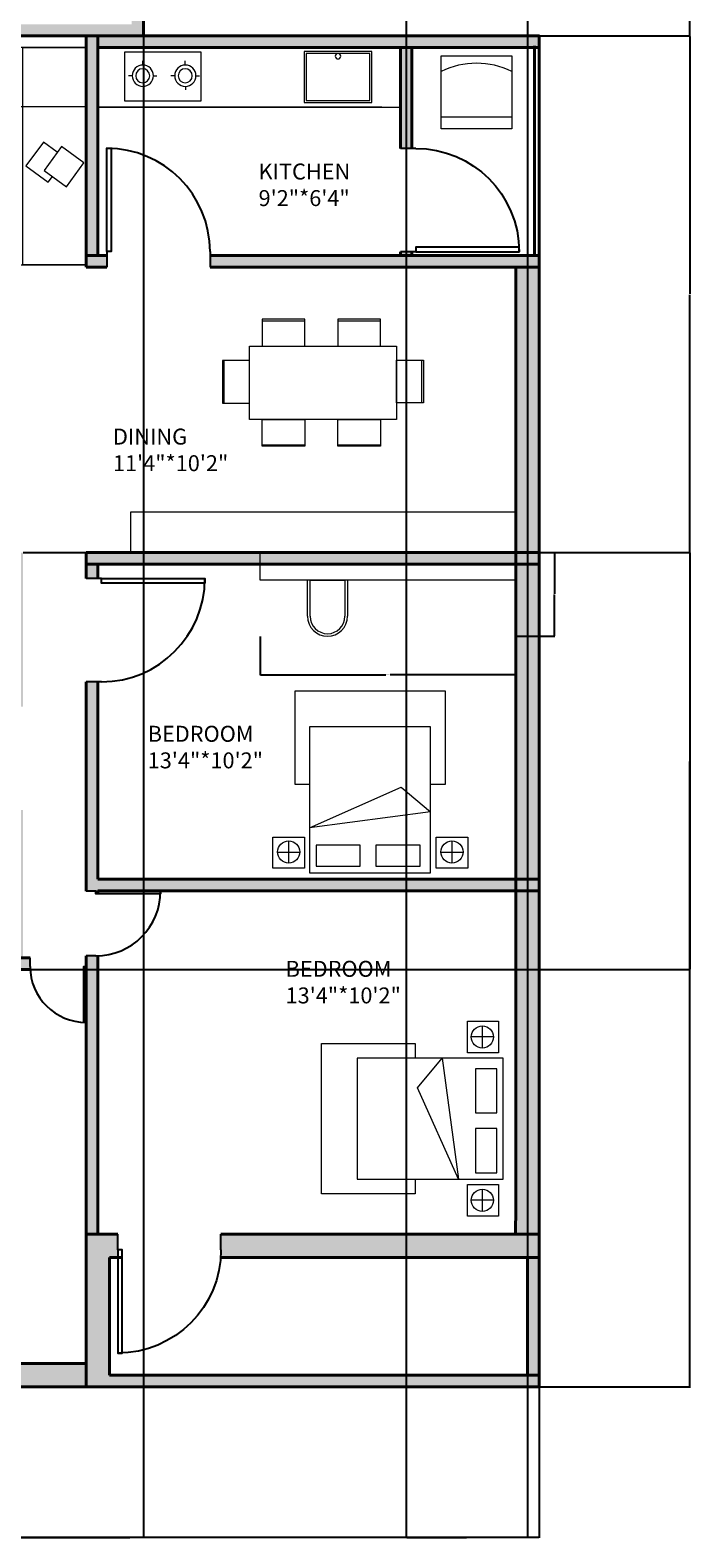
# Model space of a CAD drawing. Units: inches. Extents: x 1642 to 2399, y 1011 to 2291.
# Tile 3 of 7: x 2143 to 2399, y 1011 to 1595. Entities that reach past the tile are written whole.
import ezdxf

# ---------------------------------------------------------------- set-up
doc = ezdxf.new("R2010")
doc.units = ezdxf.units.IN
for name, color, linetype, lineweight in [('A-ANNO-DIMS', 2, 'Continuous', 18), ('A-AREA-IDEN', 7, 'Continuous', 20), ('A-DOOR', 4, 'Continuous', 25), ('A-EQPM', 8, 'Continuous', 18), ('A-FLOR-CASE', 30, 'Continuous', 18), ('A-FLOR-FIXT', 9, 'Continuous', 18), ('A-FURN', 8, 'Continuous', 18), ('A-WALL-PATT', 40, 'Continuous', 13), ('BED', 200, 'Continuous', 18), ('WALL', 40, 'Continuous', 40)]:
    doc.layers.add(name, color=color, linetype=linetype, lineweight=lineweight)
doc.styles.get("Standard").update_dxf_attribs({"font": 'arial.ttf'})
doc.dimstyles.get("Standard").update_dxf_attribs({"dimtxt": 0.18, "dimasz": 0.18, "dimexe": 0.18, "dimexo": 0.0625, "dimgap": 0.09, "dimtad": 0, "dimtih": 1, "dimtoh": 1, "dimdec": 4, "dimzin": 0, "dimdsep": 46, "dimtxsty": 'Standard', "dimcen": 0.09, "dimadec": 0, "dimazin": 0, "dimtfac": 1, "dimtdec": 4, "dimtofl": 0, "dimtmove": 0, "dimatfit": 3, "dimfxl": 1, "dimtolj": 1, "dimtzin": 0, "dimarcsym": 0})

# ---------------------------------------------------------------- blocks, each defined once
blk = doc.blocks.new('*U2')
for p, q in [((0, 0), (0, -6)), ((40, 0), (40, -6))]:
    blk.add_line(p, q)
blk.add_lwpolyline([(0, 0), (0, 40), (1.75, 40), (1.75, 0)], close=True)
blk.add_arc((0, 0), 40, 0, 90)
blk = doc.blocks.new('BED-DOUBLE-WITH-NIGHTSTANDS')
for p, q in [((8.62, 34.13), (8.62, 70.38)), ((8.62, 70.38), (66.79, 70.38)), ((66.79, 70.38), (66.79, 34.13)), ((14.22, 34.13), (8.62, 34.13)), ((14.22, 17.36), (49.69, 33.17)), ((49.69, 33.17), (61.11, 23.59)), ((66.79, 34.13), (61.11, 34.13)), ((61.11, 23.59), (14.22, 17.36)), ((6.17, 3.76), (6.17, 12.35)), ((69.41, 3.76), (69.41, 12.35)), ((1.82, 7.94), (10.42, 7.94)), ((65.06, 7.94), (73.65, 7.94))]:
    blk.add_line(p, q)
for points in [[(14.22, 0), (61.11, 0), (61.11, 56.52), (14.22, 56.52)], [(12.24, 1.79), (0, 1.79), (0, 13.82), (12.24, 13.82)], [(75.48, 1.79), (63.24, 1.79), (63.24, 13.82), (75.48, 13.82)], [(16.77, 2.51), (33.87, 2.51), (33.87, 10.66), (16.77, 10.66)], [(39.94, 2.51), (57.04, 2.51), (57.04, 10.66), (39.94, 10.66)]]:
    blk.add_lwpolyline(points, close=True)
for centre in [(6.12, 8.05), (69.36, 8.05)]:
    blk.add_circle(centre, 4.3)
blk = doc.blocks.new('TABLE-DINING-SIX-SEAT')
for p, q in [((15.31, 48.55), (31.81, 48.55)), ((44.68, 48.55), (61.18, 48.55)), ((0.59, 16.67), (0.59, 33.17)), ((77.22, 16.83), (77.22, 33.33)), ((15.31, 0.59), (31.81, 0.59)), ((44.68, 0.59), (61.18, 0.59))]:
    blk.add_line(p, q)
for points in [[(15.31, 38.77), (31.81, 38.77), (31.81, 49.15), (15.31, 49.15)], [(44.68, 38.77), (61.18, 38.77), (61.18, 49.15), (44.68, 49.15)], [(10.38, 38.77), (67.43, 38.77), (67.43, 10.38), (10.38, 10.38)], [(10.38, 16.67), (10.38, 33.17), (0, 33.17), (0, 16.67)], [(67.43, 16.83), (67.43, 33.33), (77.81, 33.33), (77.81, 16.83)], [(15.31, 10.38), (31.81, 10.38), (31.81, 0), (15.31, 0)], [(44.68, 10.38), (61.18, 10.38), (61.18, 0), (44.68, 0)]]:
    blk.add_lwpolyline(points, close=True)
blk = doc.blocks.new('SEATING-CORNER')
for points in [[(0, 84.13), (76.26, 84.13), (76.26, 61.34), (0, 61.34)], [(0, 0), (24.56, 0), (24.56, 84.13), (0, 84.13)], [(56.51, 80.66), (63.26, 71.39), (54.61, 65.09), (47.86, 74.37)], [(9.57, 45.8), (16.32, 36.53), (7.67, 30.23), (0.92, 39.51)]]:
    blk.add_lwpolyline(points, close=True)
for points in [[(58.1, 78.48), (63.51, 82.42), (70.26, 73.15), (61.61, 66.85), (60.02, 69.03)], [(11.16, 43.62), (16.57, 47.56), (23.32, 38.28), (14.67, 31.99), (13.08, 34.17)]]:
    blk.add_lwpolyline(points)
blk = doc.blocks.new('COOKTOP-TWO-BURNER')
for p, q in [((6.17, 13.89), (6.17, 15.59)), ((22.64, 13.89), (22.64, 15.59)), ((2, 9.67), (0.69, 9.67)), ((10.24, 9.72), (11.69, 9.72)), ((18.47, 9.67), (17.17, 9.67)), ((26.71, 9.72), (28.17, 9.72)), ((6.02, 5.65), (6.02, 4.35)), ((22.49, 5.65), (22.49, 4.35))]:
    blk.add_line(p, q)
blk.add_lwpolyline([(0, 18.89), (29.66, 18.89), (29.66, 0), (0, 0)], close=True)
for centre, radius in [((6.12, 9.77), 4.12), ((6.17, 9.77), 2.71), ((22.59, 9.77), 4.12), ((22.64, 9.77), 2.71)]:
    blk.add_circle(centre, radius)
blk = doc.blocks.new('SINK-KITCHEN-SINGLE')
for points in [[(0, 19.82), (26.24, 19.82), (26.24, 0), (0, 0)], [(0.83, 18.98), (25.41, 18.98), (25.41, 0.83), (0.83, 0.83)]]:
    blk.add_lwpolyline(points, close=True)
blk.add_circle((13.12, 17.93), 1.05)
blk = doc.blocks.new('UTILITY-APPLIANCE')
blk.add_line((0, 4.7), (27.35, 4.7))
blk.add_lwpolyline([(0, 28.26), (27.35, 28.26), (27.35, 0), (0, 0)], close=True)
blk.add_arc((13.68, -6.28), 31.65, 64.3994, 115.6006)
blk = doc.blocks.new('DESK-WITH-CHAIR')
blk.add_lwpolyline([(0, 32.44), (99.14, 32.44), (99.14, 21.72), (0, 21.72)], close=True)
for points in [[(18.41, 7.73), (18.41, 21.72)], [(19.41, 7.73), (19.41, 21.72), (32.87, 21.72), (32.87, 7.73)], [(33.87, 21.72), (33.87, 7.73)]]:
    blk.add_lwpolyline(points)
for radius in [7.73, 6.73]:
    blk.add_arc((26.14, 7.73), radius, 180, 0)
blk = doc.blocks.new('*D30')
at = {"layer": 'A-ANNO-DIMS', "color": 0, "lineweight": -2, "transparency": 16777216}
for p, q in [((2232.04, 1360.21), (2232.04, 1345.22)), ((2331.18, 1360.21), (2331.18, 1345.22)), ((2232.22, 1345.4), (2280.71, 1345.4)), ((2331, 1345.4), (2282.51, 1345.4))]:
    blk.add_line(p, q, dxfattribs=at)
at = {"layer": 'A-ANNO-DIMS', "color": 0, "transparency": 16777216}
for points in [[(2232.22, 1345.43), (2232.22, 1345.37), (2232.04, 1345.4)], [(2331, 1345.43), (2331, 1345.37), (2331.18, 1345.4)]]:
    blk.add_solid(points, dxfattribs=at)
at = {"layer": 'Defpoints', "color": 0, "transparency": 16777216}
for p in [(2232.04, 1360.27), (2331.18, 1360.27), (2331.18, 1345.4)]:
    blk.add_point(p, dxfattribs=at)
at = {"layer": 'A-ANNO-DIMS', "color": 0, "transparency": 16777216, "insert": (2281.61, 1345.4), "char_height": 0.18, "attachment_point": 5}
blk.add_mtext('\\A1;DESK 99 TYP.', dxfattribs=at)
blk = doc.blocks.new('*D31')
at = {"layer": 'A-ANNO-DIMS', "color": 0, "lineweight": -2, "transparency": 16777216}
for p, q in [((2331.24, 1392.71), (2346.23, 1392.71)), ((2346.05, 1392.53), (2346.05, 1376.67)), ((2346.05, 1360.45), (2346.05, 1376.31)), ((2331.24, 1360.27), (2346.23, 1360.27))]:
    blk.add_line(p, q, dxfattribs=at)
at = {"layer": 'A-ANNO-DIMS', "color": 0, "transparency": 16777216}
for points in [[(2346.02, 1392.53), (2346.08, 1392.53), (2346.05, 1392.71)], [(2346.02, 1360.45), (2346.08, 1360.45), (2346.05, 1360.27)]]:
    blk.add_solid(points, dxfattribs=at)
at = {"layer": 'Defpoints', "color": 0, "transparency": 16777216}
for p in [(2331.18, 1392.71), (2346.05, 1392.71), (2331.18, 1360.27)]:
    blk.add_point(p, dxfattribs=at)
at = {"layer": 'A-ANNO-DIMS', "color": 0, "transparency": 16777216, "insert": (2346.05, 1376.49), "char_height": 0.18, "attachment_point": 5}
blk.add_mtext('\\A1;32 TYP.', dxfattribs=at)
blk = doc.blocks.new('*D34')
at = {"layer": 'A-ANNO-DIMS', "color": 0, "lineweight": -2, "transparency": 16777216}
for p, q in [((2340.24, 1392.71), (2398.73, 1392.71)), ((2398.55, 1392.53), (2398.55, 1231.39)), ((2398.55, 1069.89), (2398.55, 1231.03)), ((2340.24, 1069.71), (2398.73, 1069.71))]:
    blk.add_line(p, q, dxfattribs=at)
at = {"layer": 'A-ANNO-DIMS', "color": 0, "transparency": 16777216}
for points in [[(2398.52, 1392.53), (2398.58, 1392.53), (2398.55, 1392.71)], [(2398.52, 1069.89), (2398.58, 1069.89), (2398.55, 1069.71)]]:
    blk.add_solid(points, dxfattribs=at)
at = {"layer": 'Defpoints', "color": 0, "transparency": 16777216}
for p in [(2340.18, 1392.71), (2398.55, 1392.71), (2340.18, 1069.71)]:
    blk.add_point(p, dxfattribs=at)
at = {"layer": 'A-ANNO-DIMS', "color": 0, "transparency": 16777216, "insert": (2398.55, 1231.21), "char_height": 0.18, "attachment_point": 5}
blk.add_mtext('\\A1;323', dxfattribs=at)
blk = doc.blocks.new('*D35')
at = {"layer": 'A-ANNO-DIMS', "color": 0, "lineweight": -2, "transparency": 16777216}
for p, q in [((2340.24, 1592.71), (2398.73, 1592.71)), ((2398.55, 1592.53), (2398.55, 1492.89)), ((2398.55, 1392.89), (2398.55, 1492.53)), ((2340.24, 1392.71), (2398.73, 1392.71))]:
    blk.add_line(p, q, dxfattribs=at)
at = {"layer": 'A-ANNO-DIMS', "color": 0, "transparency": 16777216}
for points in [[(2398.52, 1592.53), (2398.58, 1592.53), (2398.55, 1592.71)], [(2398.52, 1392.89), (2398.58, 1392.89), (2398.55, 1392.71)]]:
    blk.add_solid(points, dxfattribs=at)
at = {"layer": 'Defpoints', "color": 0, "transparency": 16777216}
for p in [(2340.18, 1592.71), (2398.55, 1592.71), (2340.18, 1392.71)]:
    blk.add_point(p, dxfattribs=at)
at = {"layer": 'A-ANNO-DIMS', "color": 0, "transparency": 16777216, "insert": (2398.55, 1492.71), "char_height": 0.18, "attachment_point": 5}
blk.add_mtext('\\A1;200', dxfattribs=at)
blk = doc.blocks.new('*D36')
at = {"layer": 'A-ANNO-DIMS', "color": 0, "lineweight": -2, "transparency": 16777216}
for p, q in [((2340.24, 1709.46), (2398.73, 1709.46)), ((2398.55, 1709.28), (2398.55, 1651.26)), ((2398.55, 1592.89), (2398.55, 1650.9)), ((2340.24, 1592.71), (2398.73, 1592.71))]:
    blk.add_line(p, q, dxfattribs=at)
at = {"layer": 'A-ANNO-DIMS', "color": 0, "transparency": 16777216}
for points in [[(2398.52, 1709.28), (2398.58, 1709.28), (2398.55, 1709.46)], [(2398.52, 1592.89), (2398.58, 1592.89), (2398.55, 1592.71)]]:
    blk.add_solid(points, dxfattribs=at)
at = {"layer": 'Defpoints', "color": 0, "transparency": 16777216}
for p in [(2340.18, 1709.46), (2398.55, 1709.46), (2340.18, 1592.71)]:
    blk.add_point(p, dxfattribs=at)
at = {"layer": 'A-ANNO-DIMS', "color": 0, "transparency": 16777216, "insert": (2398.55, 1651.08), "char_height": 0.18, "attachment_point": 5}
blk.add_mtext('\\A1;116.75', dxfattribs=at)
blk = doc.blocks.new('*D40')
at = {"layer": 'A-ANNO-DIMS', "color": 0, "lineweight": -2, "transparency": 16777216}
for p, q in [((1796.18, 1709.39), (1796.18, 1011.19)), ((2186.88, 1709.39), (2186.88, 1011.19)), ((1796.36, 1011.37), (1991.13, 1011.37)), ((2186.7, 1011.37), (1991.92, 1011.37))]:
    blk.add_line(p, q, dxfattribs=at)
at = {"layer": 'A-ANNO-DIMS', "color": 0, "transparency": 16777216}
for points in [[(1796.36, 1011.4), (1796.36, 1011.34), (1796.18, 1011.37)], [(2186.7, 1011.4), (2186.7, 1011.34), (2186.88, 1011.37)]]:
    blk.add_solid(points, dxfattribs=at)
at = {"layer": 'Defpoints', "color": 0, "transparency": 16777216}
for p in [(1796.18, 1709.46), (2186.88, 1709.46), (2186.88, 1011.37)]:
    blk.add_point(p, dxfattribs=at)
at = {"layer": 'A-ANNO-DIMS', "color": 0, "transparency": 16777216, "insert": (1991.53, 1011.37), "char_height": 0.18, "attachment_point": 5}
blk.add_mtext('\\A1;390.7', dxfattribs=at)
blk = doc.blocks.new('*D45')
at = {"layer": 'A-ANNO-DIMS', "color": 0, "lineweight": -2, "transparency": 16777216}
for p, q in [((2023.71, 1069.65), (2023.71, 1011.19)), ((2340.18, 1069.65), (2340.18, 1011.19)), ((2023.89, 1011.37), (2181.55, 1011.37)), ((2340, 1011.37), (2182.34, 1011.37))]:
    blk.add_line(p, q, dxfattribs=at)
at = {"layer": 'A-ANNO-DIMS', "color": 0, "transparency": 16777216}
for points in [[(2023.89, 1011.4), (2023.89, 1011.34), (2023.71, 1011.37)], [(2340, 1011.4), (2340, 1011.34), (2340.18, 1011.37)]]:
    blk.add_solid(points, dxfattribs=at)
at = {"layer": 'Defpoints', "color": 0, "transparency": 16777216}
for p in [(2023.71, 1069.71), (2340.18, 1069.71), (2340.18, 1011.37)]:
    blk.add_point(p, dxfattribs=at)
at = {"layer": 'A-ANNO-DIMS', "color": 0, "transparency": 16777216, "insert": (2181.95, 1011.37), "char_height": 0.18, "attachment_point": 5}
blk.add_mtext('\\A1;316.5', dxfattribs=at)
blk = doc.blocks.new('*D47')
at = {"layer": 'A-ANNO-DIMS', "color": 0, "lineweight": -2, "transparency": 16777216}
for p, q in [((2288.68, 1713.89), (2288.68, 1011.19)), ((2335.68, 1713.89), (2335.68, 1011.19)), ((2288.86, 1011.37), (2311.96, 1011.37)), ((2335.5, 1011.37), (2312.4, 1011.37))]:
    blk.add_line(p, q, dxfattribs=at)
at = {"layer": 'A-ANNO-DIMS', "color": 0, "transparency": 16777216}
for points in [[(2288.86, 1011.4), (2288.86, 1011.34), (2288.68, 1011.37)], [(2335.5, 1011.4), (2335.5, 1011.34), (2335.68, 1011.37)]]:
    blk.add_solid(points, dxfattribs=at)
at = {"layer": 'Defpoints', "color": 0, "transparency": 16777216}
for p in [(2288.68, 1713.96), (2335.68, 1713.96), (2335.68, 1011.37)]:
    blk.add_point(p, dxfattribs=at)
at = {"layer": 'A-ANNO-DIMS', "color": 0, "transparency": 16777216, "insert": (2312.18, 1011.37), "char_height": 0.18, "attachment_point": 5}
blk.add_mtext('\\A1;47', dxfattribs=at)
blk = doc.blocks.new('*D49')
at = {"layer": 'A-ANNO-DIMS', "color": 0, "lineweight": -2, "transparency": 16777216}
for p, q in [((2140.3, 1392.71), (2398.73, 1392.71)), ((2398.55, 1392.53), (2398.55, 1312.16)), ((2398.55, 1231.42), (2398.55, 1311.79)), ((2135.24, 1231.24), (2398.73, 1231.24))]:
    blk.add_line(p, q, dxfattribs=at)
at = {"layer": 'A-ANNO-DIMS', "color": 0, "transparency": 16777216}
for points in [[(2398.52, 1392.53), (2398.58, 1392.53), (2398.55, 1392.71)], [(2398.52, 1231.42), (2398.58, 1231.42), (2398.55, 1231.24)]]:
    blk.add_solid(points, dxfattribs=at)
at = {"layer": 'Defpoints', "color": 0, "transparency": 16777216}
for p in [(2140.24, 1392.71), (2135.18, 1231.24), (2398.55, 1231.24)]:
    blk.add_point(p, dxfattribs=at)
at = {"layer": 'A-ANNO-DIMS', "color": 0, "transparency": 16777216, "insert": (2398.55, 1311.98), "char_height": 0.18, "attachment_point": 5}
blk.add_mtext('\\A1;161.46', dxfattribs=at)

msp = doc.modelspace()

# ---------------------------------------------------------------- hatches: boundary and pattern name
at = {"layer": 'A-WALL-PATT'}
h = msp.add_hatch(color=256, dxfattribs=at)
h.dxf.hatch_style = 1
h.paths.add_polyline_path([(2340.1804, 2185.4562), (2211.0983, 2185.4562, -0.01876983), (2211.211, 2182.4562), (2211.211, 2176.4562), (2331.211, 2176.4562), (2331.211, 2043.4562), (2171.211, 2043.4562), (2171.211, 2038.9562), (2331.211, 2038.9562), (2331.211, 1916.9562), (2171.211, 1916.9562), (2171.211, 1918.9365), (2166.711, 1918.9365), (2166.711, 1912.4562), (2340.1804, 1912.4562)])
h.paths.add_polyline_path([(2171.211, 2043.4562), (2171.211, 2043.9025), (2170.5217, 2043.9025), (2166.711, 2043.9025), (2166.711, 2038.9562), (2166.711, 1958.9365), (2171.211, 1958.9365)], flags=17)
h.paths.add_polyline_path([(2129.211, 1971.5979), (2124.711, 1971.5979), (2124.711, 1918.4562), (2067.711, 1918.4562), (2067.711, 1913.9562), (2129.211, 1913.9562)])
h.paths.add_polyline_path([(2067.711, 2015.4562), (2124.711, 2015.4562), (2124.711, 2019.9562), (2058.711, 2019.9562), (2058.711, 2015.4562), (2058.711, 1922.9562), (1982.211, 1922.9562), (1982.211, 2015.4562), (1982.211, 2019.9562), (1916.211, 2019.9562), (1916.211, 2070.9562), (1911.711, 2070.9562), (1911.711, 2015.4562), (1911.711, 2012.302), (1916.211, 2012.302), (1916.211, 2015.4562), (1973.211, 2015.4562), (1973.211, 1918.4562), (1973.211, 1913.9562), (2017.1804, 1913.9562), (2067.711, 1913.9562), (2067.711, 1918.4562)])
h.paths.add_polyline_path([(2131.1386, 2075.4562), (2118.1934, 2075.4562), (2118.1934, 2070.9562), (2131.1386, 2070.9562)], flags=17)
h.paths.add_polyline_path([(1918.8034, 2075.4562), (1909.4956, 2075.4562), (1909.4956, 2070.9562), (1918.8034, 2070.9562)], flags=17)
h.paths.add_polyline_path([(1874.211, 2029.9562), (1869.711, 2029.9562), (1869.711, 1960.7404), (1874.211, 1960.7404)], flags=17)
h.paths.add_polyline_path([(1916.211, 1972.302), (1911.711, 1972.302), (1911.711, 1918.4562), (1916.211, 1918.4562)], flags=17)
h.paths.add_polyline_path([(2340.1804, 1912.4562), (2331.1804, 1912.4562), (2331.1804, 1794.4562), (2210.1804, 1794.4562), (2210.1804, 1789.9562), (2279.6804, 1789.9562), (2340.1804, 1789.9562)])
h.paths.add_polyline_path([(2288.6804, 1789.9562), (2279.6804, 1789.9562), (2279.6804, 1785.0846), (2285.6804, 1785.0846), (2288.6804, 1785.0846)], flags=17)
h.paths.add_polyline_path([(2169.6804, 1789.9562), (2170.1804, 1789.9562), (2170.1804, 1794.4562), (2165.1804, 1794.4562), (2165.1804, 1713.9562), (2165.1804, 1709.4562), (2279.6804, 1709.4562), (2279.6804, 1718.4562), (2169.6804, 1718.4562)])
h.paths.add_polyline_path([(2288.6804, 1745.1973, -0.01876983), (2285.6804, 1745.0846), (2279.6804, 1745.0846), (2279.6804, 1709.4562), (2340.1804, 1709.4562), (2340.1804, 1789.9562), (2335.6804, 1789.9562), (2335.6804, 1713.9562), (2288.6804, 1713.9562)])
h.paths.add_polyline_path([(2165.1804, 1713.9562), (2140.6229, 1713.9562), (2088.923, 1713.9562), (2069.7509, 1713.9562), (2060.4457, 1713.9562), (2060.4457, 1709.4562), (2165.1804, 1709.4562)])
h.paths.add_polyline_path([(2020.4457, 1713.9562), (2017.1804, 1713.9562), (2012.6804, 1713.9562), (2009.1946, 1713.9562), (2009.1946, 1709.4562), (2020.4457, 1709.4562)])
h.paths.add_polyline_path([(1969.1946, 1713.9562), (1864.6804, 1713.9562), (1864.6804, 1798.9562), (1860.1804, 1798.9562), (1860.1804, 1792.9562), (1860.1804, 1752.9562), (1860.1804, 1718.4562), (1750.1804, 1718.4562), (1750.1804, 1749.2419), (1744.1804, 1749.2419, -0.01876983), (1741.1804, 1749.3546), (1741.1804, 1709.4562), (1969.1946, 1709.4562)])
h.paths.add_polyline_path([(1741.1804, 1803.4562), (1700.711, 1803.4562), (1700.711, 1794.4562), (1741.1804, 1794.4562)])
h.paths.add_polyline_path([(1820.1804, 1798.9562), (1741.1804, 1798.9562), (1741.1804, 1794.4562), (1741.1804, 1790.0365), (1741.1804, 1789.2419), (1744.1804, 1789.2419), (1750.1804, 1789.2419), (1750.1804, 1794.4562), (1820.1804, 1794.4562)], flags=17)
h.paths.add_polyline_path([(1800.6804, 1709.4562), (1796.1804, 1709.4562), (1796.1804, 1592.7078), (1978.9325, 1592.7078), (1978.9325, 1597.2078), (1800.6804, 1597.2078)])
h.paths.add_polyline_path([(2097.0678, 1709.4562), (2088.0678, 1709.4562), (2088.0678, 1599.6874), (2088.0678, 1597.2078), (2097.0678, 1597.2078)], flags=17)
h.paths.add_polyline_path([(2186.8766, 1709.4562), (2182.3766, 1709.4562), (2182.3766, 1597.2078), (2071.4624, 1597.2078), (2071.4624, 1592.7078), (2186.8766, 1592.7078)])
h.paths.add_polyline_path([(2078.1934, 2075.4562), (2022.711, 2075.4562), (2022.711, 2223.4562), (2166.711, 2223.4562), (2166.711, 2075.4562), (2166.711, 2070.9562), (2171.211, 2070.9562), (2171.211, 2138.8919), (2171.211, 2227.9562), (2335.711, 2227.9562), (2335.711, 2185.4562), (2340.1804, 2185.4562), (2340.1804, 2232.4562), (1874.211, 2232.4562), (1874.211, 2223.4562), (2018.211, 2223.4562), (2018.211, 2075.4562), (1958.8034, 2075.4562), (1958.8034, 2070.9562), (2018.211, 2070.9562), (2018.211, 2019.9562), (1982.211, 2019.9562), (1982.211, 2015.4562), (1982.211, 2010.9562), (2058.711, 2010.9562), (2058.711, 2015.4562), (2058.711, 2019.9562), (2022.711, 2019.9562), (2022.711, 2070.9562), (2078.1934, 2070.9562)])
h.paths.add_polyline_path([(1874.211, 2171.9562), (1874.211, 2176.4562), (1861.9371, 2176.4562), (1861.9371, 2173.4562), (1861.9371, 2167.4562), (1869.711, 2167.4562), (1869.711, 2069.7602), (1874.211, 2069.7602)], flags=17)
h.paths.add_polyline_path([(1705.211, 2227.9562), (1865.211, 2227.9562), (1865.211, 2176.4562), (1874.211, 2176.4562), (1874.211, 2232.4562), (1700.711, 2232.4562), (1700.711, 2176.4562), (1705.211, 2176.4562)])
h.paths.add_polyline_path([(1709.711, 2167.4562), (1821.9371, 2167.4562), (1821.9371, 2173.4562, -0.01876983), (1822.0498, 2176.4562), (1700.711, 2176.4562), (1700.711, 1913.9562), (1860.1804, 1913.9562), (1864.6804, 1913.9562), (1973.211, 1913.9562), (1973.211, 1918.4562), (1916.211, 1918.4562), (1874.211, 1918.4562), (1874.211, 1920.7404), (1869.711, 1920.7404), (1869.711, 1918.4562), (1860.1804, 1918.4562), (1709.711, 1918.4562), (1709.711, 2029.9562), (1874.211, 2029.9562), (1874.211, 2037.0364), (1869.711, 2037.0364), (1869.711, 2034.4562), (1709.711, 2034.4562)])
h.paths.add_polyline_path([(2017.1804, 1913.9562), (2012.6804, 1913.9562), (2012.6804, 1713.9562), (2017.1804, 1713.9562)])
h.paths.add_polyline_path([(1952.4341, 2110.3716), (2000.4134, 2110.3716), (2000.4134, 2133.4189), (1952.4341, 2133.4189)], flags=25)
h.paths.add_polyline_path([(2042.3983, 2110.7121), (2090.3775, 2110.7121), (2090.3775, 2133.7594), (2042.3983, 2133.7594)], flags=25)
h.paths.add_polyline_path([(2201.7332, 2091.8715), (2249.7125, 2091.8715), (2249.7125, 2114.9188), (2201.7332, 2114.9188)], flags=25)
h.paths.add_polyline_path([(1805.186, 2077.6915), (1853.1653, 2077.6915), (1853.1653, 2100.7388), (1805.186, 2100.7388)], flags=25)
h.paths.add_polyline_path([(1794.8897, 1974.6584), (1842.869, 1974.6584), (1842.869, 1997.7057), (1794.8897, 1997.7057)], flags=25)
h.paths.add_polyline_path([(2229.1796, 2204.4209), (2315.1362, 2204.4209), (2315.1362, 2217.1488), (2229.1796, 2217.1488)], flags=25)
h.paths.add_polyline_path([(1715.2159, 2199.5328), (1801.1724, 2199.5328), (1801.1724, 2212.2607), (1715.2159, 2212.2607)], flags=25)
h.paths.add_polyline_path([(2230.7681, 1755.7109), (2271.7283, 1755.7109), (2271.7283, 1778.7582), (2230.7681, 1778.7582)], flags=25)
h.paths.add_polyline_path([(1763.4713, 1764.1742), (1804.4315, 1764.1742), (1804.4315, 1787.2215), (1763.4713, 1787.2215)], flags=25)
h.paths.add_polyline_path([(2076.2643, 1955.0495), (2111.326, 1955.0495), (2111.326, 1978.0968), (2076.2643, 1978.0968)], flags=25)
h.paths.add_polyline_path([(1932.854, 1956.1217), (1967.9158, 1956.1217), (1967.9158, 1979.169), (1932.854, 1979.169)], flags=25)
h.paths.add_polyline_path([(2048.1203, 2031.6107), (2083.1821, 2031.6107), (2083.1821, 2054.658), (2048.1203, 2054.658)], flags=25)
h.paths.add_polyline_path([(2163.5754, 1863.7569), (2208.2347, 1863.7569), (2208.2347, 1886.8042), (2163.5754, 1886.8042)], flags=9)
h.paths.add_polyline_path([(2039.9286, 1809.0957), (2084.5879, 1809.0957), (2084.5879, 1832.143), (2039.9286, 1832.143)], flags=9)
h.paths.add_polyline_path([(1901.0045, 1814.0452), (1945.6638, 1814.0452), (1945.6638, 1837.0925), (1901.0045, 1837.0925)], flags=9)
h.paths.add_polyline_path([(1833.7282, 1852.5627), (1878.3875, 1852.5627), (1878.3875, 1875.61), (1833.7282, 1875.61)], flags=9)
h.paths.add_polyline_path([(2219.1375, 1926.2139), (2267.1167, 1926.2139), (2267.1167, 1949.2612), (2219.1375, 1949.2612)], flags=25)
h.paths.add_polyline_path([(1956.9598, 2029.7735), (1992.0216, 2029.7735), (1992.0216, 2052.8208), (1956.9598, 2052.8208)], flags=25)
h.paths.add_polyline_path([(2229.3, 1523.3399), (2270.2602, 1523.3399), (2270.2602, 1546.3872), (2229.3, 1546.3872)], flags=9)
h.paths.add_polyline_path([(1772.3039, 1526.9922), (1813.2641, 1526.9922), (1813.2641, 1550.0394), (1772.3039, 1550.0394)], flags=9)
h.paths.add_polyline_path([(2172.587, 1420.6999), (2217.2463, 1420.6999), (2217.2463, 1443.7472), (2172.587, 1443.7472)], flags=9)
h.paths.add_polyline_path([(1814.3549, 1422.215), (1859.0143, 1422.215), (1859.0143, 1445.2623), (1814.3549, 1445.2623)], flags=9)
h.paths.add_polyline_path([(2186.0372, 1305.6227), (2234.0165, 1305.6227), (2234.0165, 1328.67), (2186.0372, 1328.67)], flags=9)
h.paths.add_polyline_path([(1756.747, 1349.0694), (1804.7263, 1349.0694), (1804.7263, 1372.1167), (1756.747, 1372.1167)], flags=9)
h.paths.add_polyline_path([(2239.449, 1214.6184), (2287.4282, 1214.6184), (2287.4282, 1237.6657), (2239.449, 1237.6657)], flags=9)
h.paths.add_polyline_path([(1767.104, 1213.8348), (1815.0832, 1213.8348), (1815.0832, 1236.8821), (1767.104, 1236.8821)], flags=9)
h.paths.add_polyline_path([(2046.6809, 1183.6854), (2094.6602, 1183.6854), (2094.6602, 1206.7327), (2046.6809, 1206.7327)], flags=9)
h.paths.add_polyline_path([(1947.2155, 1183.6854), (1995.1948, 1183.6854), (1995.1948, 1206.7327), (1947.2155, 1206.7327)], flags=9)
h.paths.add_polyline_path([(1959.3556, 1258.7871), (1994.4174, 1258.7871), (1994.4174, 1281.8344), (1959.3556, 1281.8344)], flags=9)
h.paths.add_polyline_path([(2049.6419, 1248.9629), (2084.7036, 1248.9629), (2084.7036, 1272.0102), (2049.6419, 1272.0102)], flags=9)
h.paths.add_polyline_path([(2092.7532, 1327.4852), (2127.815, 1327.4852), (2127.815, 1350.5325), (2092.7532, 1350.5325)], flags=9)
h.paths.add_polyline_path([(1944.9358, 1327.4852), (1979.9976, 1327.4852), (1979.9976, 1350.5325), (1944.9358, 1350.5325)], flags=9)
h.paths.add_polyline_path([(1974.5055, 1650.063), (2006.3695, 1650.063), (2006.3695, 1662.7909), (1974.5055, 1662.7909)], flags=9)
h = msp.add_hatch(color=256, dxfattribs=at)
h.dxf.hatch_style = 1
h.paths.add_polyline_path([(2078.7415, 1388.2078), (2028.211, 1388.2078), (2028.211, 1383.7078), (2069.7415, 1383.7078), (2069.7415, 1291.2078), (2069.7415, 1286.7078), (2135.7415, 1286.7078), (2135.7415, 1291.2078), (2078.7415, 1291.2078)])
h.paths.add_polyline_path([(1993.2415, 1383.7078), (2023.711, 1383.7078), (2023.711, 1388.2078), (1984.2415, 1388.2078), (1984.2415, 1291.2078), (1927.2415, 1291.2078), (1927.2415, 1296.6705), (1922.7415, 1296.6705), (1922.7415, 1291.2078), (1922.7415, 1235.7078), (1927.2415, 1235.7078), (1927.2415, 1237.2428), (1927.2415, 1277.2428), (1927.2415, 1286.7078), (1993.2415, 1286.7078), (1993.2415, 1291.2078)])
h.paths.add_polyline_path([(1927.2415, 1388.2078), (1922.7415, 1388.2078), (1922.7415, 1336.6705), (1927.2415, 1336.6705)])
h.paths.add_polyline_path([(1984.2415, 1392.7078), (1922.7415, 1392.7078), (1922.7415, 1388.2078), (1984.2415, 1388.2078)])
h.paths.add_polyline_path([(2023.711, 1392.7078), (1984.2415, 1392.7078), (1984.2415, 1388.2078), (2023.711, 1388.2078)])
h.paths.add_polyline_path([(2078.7415, 1392.7078), (2028.211, 1392.7078), (2028.211, 1388.2078), (2078.7415, 1388.2078)])
h.paths.add_polyline_path([(2140.2415, 1392.7078), (2078.7415, 1392.7078), (2078.7415, 1388.2078), (2135.7415, 1388.2078), (2140.2415, 1388.2078)])
h.paths.add_polyline_path([(2028.211, 1592.7078), (2023.711, 1592.7078), (2023.711, 1392.7078), (2028.211, 1392.7078)])
h.paths.add_polyline_path([(2028.211, 1388.2078), (2023.711, 1388.2078), (2023.711, 1383.7078), (2028.211, 1383.7078)])
h.paths.add_polyline_path([(2028.211, 1392.7078), (2023.711, 1392.7078), (2023.711, 1388.2078), (2028.211, 1388.2078)])
h.paths.add_polyline_path([(2140.2415, 1388.2078), (2135.7415, 1388.2078), (2135.7415, 1332.9578), (2140.2415, 1332.9578)])
h.paths.add_polyline_path([(2069.7415, 1291.2078), (2069.7415, 1295.7078), (2028.211, 1295.7078), (2023.711, 1295.7078), (1993.2415, 1295.7078), (1993.2415, 1291.2078), (1993.2415, 1286.7078), (2029.2415, 1286.7078), (2047.9002, 1286.7078), (2053.9738, 1286.7078), (2069.7415, 1286.7078)])
h.paths.add_polyline_path([(2140.2415, 1291.2078), (2140.2415, 1292.9578), (2135.7415, 1292.9578), (2135.7415, 1269.1323), (2135.7415, 1235.7078), (2140.2415, 1235.7078)])
h.paths.add_polyline_path([(2232.0378, 1392.7078), (2164.6804, 1392.7078), (2164.6804, 1388.2078), (2232.0378, 1388.2078)])
h.paths.add_polyline_path([(2331.1804, 1392.7078), (2232.0378, 1392.7078), (2232.0378, 1388.2078), (2331.1804, 1388.2078)])
h.paths.add_polyline_path([(2340.1804, 1392.7078), (2331.1804, 1392.7078), (2331.1804, 1388.2078), (2340.1804, 1388.2078)])
h.paths.add_polyline_path([(2340.1804, 1388.2078), (2331.1804, 1388.2078), (2331.1804, 1381.9887), (2331.1804, 1266.2078), (2340.1804, 1266.2078)])
h.paths.add_polyline_path([(2331.1804, 1266.2078), (2169.1804, 1266.2078), (2169.1804, 1342.6266), (2164.6804, 1342.6266), (2164.6804, 1266.2078), (2164.6804, 1261.6393), (2168.4442, 1261.6393), (2169.1804, 1261.6393), (2169.1804, 1261.7078), (2331.1804, 1261.7078)])
h.paths.add_polyline_path([(2340.1804, 1266.2078), (2331.1804, 1266.2078), (2331.1804, 1261.7078), (2340.1804, 1261.7078)])
h.paths.add_polyline_path([(2340.1804, 1503.2078), (2331.1804, 1503.2078), (2331.1804, 1392.7078), (2340.1804, 1392.7078)])
h.paths.add_polyline_path([(2340.1804, 1261.7078), (2331.1804, 1261.7078), (2331.1804, 1139.2078), (2331.0462, 1128.7078), (2340.1804, 1128.7078)])
h.paths.add_polyline_path([(2169.1804, 1236.5578, -0.00733557), (2168.4442, 1236.547), (2164.6804, 1236.547), (2164.6804, 1128.7078), (2169.1804, 1128.7078)])
h.paths.add_polyline_path([(2095.1813, 1235.7078), (2028.211, 1235.7078), (2028.211, 1231.2428), (2095.1813, 1231.2428)])
h.paths.add_polyline_path([(2028.211, 1286.7078), (2023.711, 1286.7078), (2023.711, 1235.7078), (2028.211, 1235.7078)])
h.paths.add_polyline_path([(2028.211, 1235.7078), (2023.711, 1235.7078), (2023.711, 1231.2428), (2028.211, 1231.2428)])
h.paths.add_polyline_path([(2023.711, 1235.7078), (1967.2415, 1235.7078), (1967.2415, 1231.2428), (2023.711, 1231.2428)])
h.paths.add_polyline_path([(2028.211, 1231.2428), (2023.711, 1231.2428), (2023.711, 1078.7078), (2028.211, 1078.7078)])
h.paths.add_polyline_path([(1866.711, 1074.2078), (1705.211, 1074.2078), (1705.211, 1119.7078), (1700.711, 1119.7078), (1700.711, 1069.7078), (1866.711, 1069.7078)])
h.paths.add_polyline_path([(2023.711, 1078.7078), (1875.711, 1078.7078), (1875.711, 1074.2078), (1875.711, 1069.7078), (2023.711, 1069.7078)])
h.paths.add_polyline_path([(2028.211, 1078.7078), (2023.711, 1078.7078), (2023.711, 1069.7078), (2028.211, 1069.7078)])
h.paths.add_polyline_path([(2164.6804, 1078.7078), (2028.211, 1078.7078), (2028.211, 1069.7078), (2164.6804, 1069.7078), (2164.6804, 1074.2078)])
h = msp.add_hatch(color=256, dxfattribs=at)
h.dxf.hatch_style = 1
h.paths.add_polyline_path([(1875.711, 1343.4643), (1871.211, 1343.4643), (1871.211, 1266.2078), (1709.711, 1266.2078), (1709.711, 1388.2078), (1700.711, 1388.2078), (1700.711, 1261.7078), (1709.711, 1261.7078), (1875.711, 1261.7078)])
h.paths.add_polyline_path([(1761.211, 1583.7078), (1761.211, 1588.2078), (1761.211, 1592.7078), (1700.711, 1592.7078), (1700.711, 1388.2078), (1709.711, 1388.2078), (1808.8535, 1388.2078), (1871.211, 1388.2078), (1871.211, 1397.2078), (1709.711, 1397.2078), (1709.711, 1503.2078), (1761.211, 1503.2078), (1825.4443, 1503.2078), (1825.4443, 1507.7078), (1761.211, 1507.7078), (1705.211, 1507.7078), (1705.211, 1516.7078), (1705.211, 1588.2078), (1752.211, 1588.2078), (1752.211, 1516.7078), (1752.211, 1507.7078), (1761.211, 1507.7078)])
h.paths.add_polyline_path([(1875.711, 1592.7078), (1761.211, 1592.7078), (1761.211, 1588.2078), (1761.211, 1583.7078), (1871.211, 1583.7078), (1871.211, 1507.7078), (1871.211, 1503.2078), (1875.711, 1503.2078), (1875.711, 1551.7879), (1875.711, 1583.7078)])
h.paths.add_polyline_path([(1823.9074, 1128.7078), (1709.711, 1128.7078), (1709.711, 1261.7078), (1700.711, 1261.7078), (1700.711, 1119.7078), (1705.211, 1119.7078), (1709.711, 1119.7078), (1824.02, 1119.7078, -0.01876983), (1823.9074, 1122.7078)])
h.paths.add_polyline_path([(1875.711, 1236.6154), (1871.9471, 1236.6154, -0.00733557), (1871.211, 1236.6262), (1871.211, 1128.7078), (1863.9074, 1128.7078), (1863.9074, 1122.7078), (1863.9074, 1119.7078), (1866.711, 1119.7078), (1866.711, 1074.2078), (1866.711, 1069.7078), (1875.711, 1069.7078), (1875.711, 1074.2078), (1875.711, 1128.7078)])
h.paths.add_polyline_path([(2173.6804, 1119.7078), (2176.9153, 1119.7078), (2176.9153, 1122.7078), (2176.9153, 1128.7078), (2164.6804, 1128.7078), (2164.6804, 1074.2078), (2164.6804, 1069.7078), (2340.1804, 1069.7078), (2340.1804, 1074.2078), (2335.6804, 1074.2078), (2180.1804, 1074.2078), (2173.6804, 1074.2078)])
h.paths.add_polyline_path([(2340.1804, 1128.7078), (2216.9153, 1128.7078), (2216.9153, 1122.7078, -0.01876983), (2216.8027, 1119.7078), (2340.1804, 1119.7078)], flags=17)
h.paths.add_polyline_path([(2340.1804, 1119.7078), (2335.6804, 1119.7078), (2335.6804, 1074.2078), (2340.1804, 1074.2078)], flags=17)
h.paths.add_polyline_path([(2169.1804, 1592.7078), (2164.6804, 1592.7078), (2164.6804, 1507.7078), (2169.1804, 1507.7078)])
h.paths.add_polyline_path([(2340.1804, 1592.7078), (2169.1804, 1592.7078), (2169.1804, 1588.2078), (2340.1804, 1588.2078)])
h.paths.add_polyline_path([(2340.1804, 1507.7078), (2212.6763, 1507.7078), (2212.6763, 1503.2078), (2340.1804, 1503.2078)])
h.paths.add_polyline_path([(2290.8982, 1588.2078), (2286.3982, 1588.2078), (2286.3982, 1549.1888), (2290.8982, 1549.1888)])
h = msp.add_hatch(color=256, dxfattribs=at)
h.dxf.hatch_style = 1
h.paths.add_polyline_path([(1871.211, 1507.7078), (1865.4443, 1507.7078), (1865.4443, 1503.2078), (1871.211, 1503.2078)])
h.paths.add_polyline_path([(2172.6763, 1507.7078), (2164.6804, 1507.7078), (2164.6804, 1504.0795), (2164.6804, 1503.2078), (2172.6763, 1503.2078)])
h.paths.add_polyline_path([(2290.8982, 1509.1888), (2286.3982, 1509.1888), (2286.3982, 1507.7078), (2290.8982, 1507.7078)])
h.paths.add_polyline_path([(2169.1804, 1388.2078), (2164.6804, 1388.2078), (2164.6804, 1382.6266), (2169.1804, 1382.6266)])
h.paths.add_polyline_path([(2142.989, 1235.7078), (2135.7415, 1235.7078), (2135.1813, 1235.7078), (2135.1813, 1231.2428), (2143.0228, 1231.2428, -0.01396842), (2142.989, 1232.4541)])
h.paths.add_polyline_path([(1927.2415, 1235.7078), (1919.2515, 1235.7078), (1919.2515, 1231.2428), (1926.6813, 1231.2428), (1927.2415, 1231.2428)])
h.paths.add_polyline_path([(1879.2515, 1235.7078), (1875.711, 1235.7078), (1875.711, 1231.2428), (1879.2515, 1231.2428)])

# ---------------------------------------------------------------- linework, layer by layer
at = {"layer": 'A-FLOR-CASE'}
for p, q in [((2169.1804, 1592.7078), (2169.1804, 1568.7078)), ((2279.1804, 1565.1385), (2169.1804, 1565.1385)), ((2169.1804, 1565.1385), (2286.3982, 1565.1385)), ((2181.9457, 1392.7078), (2181.9457, 1408.5123)), ((2181.9457, 1408.5123), (2331.1804, 1408.5123))]:
    msp.add_line(p, q, dxfattribs=at)
at = {"layer": 'A-FURN'}
msp.add_lwpolyline([(2164.6804, 1588.2078), (2073.8807, 1588.2078), (2073.8807, 1504.0795), (2164.6804, 1504.0795)], close=True, dxfattribs=at)
at = {"layer": 'WALL'}
for p, q in [((2186.8766, 1709.4562), (2186.8766, 1592.7078)), ((2071.4624, 1592.7078), (2186.8766, 1592.7078)), ((2164.6804, 1507.7078), (2164.6804, 1592.7078)), ((2169.1804, 1507.7078), (2169.1804, 1592.7078)), ((2169.1804, 1588.2078), (2340.1804, 1588.2078)), ((2286.3982, 1588.2078), (2286.3982, 1549.1888)), ((2290.8982, 1588.2078), (2290.8982, 1549.1888)), ((2338.2991, 1588.8867), (2338.2991, 1508.3867)), ((2340.1804, 1588.2078), (2340.1804, 1507.7078)), ((2164.6804, 1507.7078), (2172.6763, 1507.7078)), ((2164.6804, 1507.7078), (2164.6804, 1503.2078)), ((2212.6763, 1507.7078), (2340.1804, 1507.7078)), ((2286.3982, 1509.1888), (2286.3982, 1507.7078)), ((2290.8982, 1509.1888), (2290.8982, 1507.7078)), ((2164.6804, 1503.2078), (2172.6763, 1503.2078)), ((2212.6763, 1503.2078), (2340.1804, 1503.2078)), ((2331.1804, 1266.2078), (2331.1804, 1503.2078)), ((2340.1804, 1266.2078), (2340.1804, 1503.2078)), ((2164.6804, 1388.2078), (2164.6804, 1392.7078)), ((2164.6804, 1392.7078), (2340.1804, 1392.7078)), ((2164.6804, 1382.6266), (2164.6804, 1388.2078)), ((2164.6804, 1388.2078), (2340.1804, 1388.2078)), ((2169.1804, 1382.6266), (2169.1804, 1388.2078)), ((2164.6804, 1266.2078), (2164.6804, 1342.6266)), ((2169.1804, 1266.2078), (2169.1804, 1342.6266)), ((2164.6804, 1261.6393), (2164.6804, 1266.2078)), ((2169.1804, 1266.2078), (2340.1804, 1266.2078)), ((2169.1804, 1261.7078), (2340.1804, 1261.7078)), ((2169.1804, 1260.5415), (2169.1804, 1261.7078)), ((2331.1804, 1139.2078), (2331.1804, 1266.2078)), ((2135.7415, 1235.7078), (2142.989, 1235.7078)), ((2164.6804, 1128.7078), (2164.6804, 1236.547)), ((2169.1804, 1128.7078), (2169.1804, 1236.5578)), ((2135.1813, 1231.2428), (2143.0228, 1231.2428)), ((2163.7314, 1231.2428), (2164.6804, 1231.2428)), ((2340.1804, 1139.2078), (2340.1804, 1223.1625)), ((2331.1804, 1139.2078), (2331.0462, 1128.7078)), ((2164.6804, 1128.7078), (2176.9153, 1128.7078)), ((2164.6804, 1074.2078), (2164.6804, 1128.7078)), ((2216.9153, 1128.7078), (2340.1804, 1128.7078)), ((2340.1804, 1074.2078), (2340.1804, 1130.2078)), ((2173.6804, 1119.7078), (2178.6653, 1119.7078)), ((2173.6804, 1074.2078), (2173.6804, 1119.7078)), ((2216.8027, 1119.7078), (2340.1804, 1119.7078)), ((2335.6804, 1074.2078), (2335.6804, 1119.7078)), ((1875.711, 1078.7078), (2164.6804, 1078.7078)), ((2164.6804, 1074.2078), (2164.6804, 1069.7078)), ((2335.6804, 1074.2078), (2173.6804, 1074.2078)), ((2340.1804, 1074.2078), (2180.1804, 1074.2078)), ((2340.1804, 1074.2078), (2335.6804, 1074.2078)), ((2340.1804, 1069.7078), (2340.1804, 1074.2078)), ((1875.711, 1069.7078), (2164.6804, 1069.7078))]:
    msp.add_line(p, q, dxfattribs=at)
msp.add_lwpolyline([(2071.4624, 1592.7078), (2340.1804, 1592.7078), (2340.1804, 1069.7078), (1700.711, 1069.7078), (1700.711, 1592.7078), (1978.9325, 1592.7078)], dxfattribs=at)

# ---------------------------------------------------------------- block references
at = {"layer": 'A-DOOR'}
msp.add_blockref('*U2', (2172.6763, 1509.2078), dxfattribs=at)
at = {"layer": 'A-DOOR', "xscale": -1}
for p, rotation in [((2292.3982, 1509.1888), 270), ((2176.9153, 1122.7078), 180)]:
    msp.add_blockref('*U2', p, dxfattribs=dict(at, rotation=rotation))
at = {"layer": 'A-DOOR', "rotation": 270}
msp.add_blockref('*U2', (2170.6804, 1382.6266), dxfattribs=at)
at = {"layer": 'A-DOOR'}
for p, xscale, yscale, zscale, rotation in [((2168.4442, 1261.6393), 0.6273086553554587, 0.6273086553554587, 0.6273086553554587, 270), ((2164.6804, 1232.4541), 0.5422858332505319, 0.5422858332505319, 0.5422858332505319, 180)]:
    msp.add_blockref('*U2', p, dxfattribs=dict(at, xscale=xscale, yscale=yscale, zscale=zscale, rotation=rotation))
at = {"layer": 'A-EQPM', "extrusion": (0, 0, -1), "zscale": -1}
msp.add_blockref('COOKTOP-TWO-BURNER', (-2209.2344, 1567.5376), dxfattribs=at)
at = {"layer": 'A-EQPM'}
msp.add_blockref('UTILITY-APPLIANCE', (2302.2103, 1556.7494), dxfattribs=at)
at = {"layer": 'A-FLOR-FIXT', "extrusion": (0, 0, -1), "zscale": -1}
msp.add_blockref('SINK-KITCHEN-SINGLE', (-2275.3657, 1566.9353), dxfattribs=at)
at = {"layer": 'A-FURN', "extrusion": (0, 0, -1), "zscale": -1}
msp.add_blockref('SEATING-CORNER', (-2164.6804, 1504.0795), dxfattribs=at)
at = {"layer": 'A-FURN'}
for name, p in [('TABLE-DINING-SIX-SEAT', (2217.527, 1433.8458)), ('DESK-WITH-CHAIR', (2232.0378, 1360.2723))]:
    msp.add_blockref(name, p, dxfattribs=at)
at = {"layer": 'BED'}
msp.add_blockref('BED-DOUBLE-WITH-NIGHTSTANDS', (2237.0179, 1268.7212), dxfattribs=at)
at = {"layer": 'BED', "rotation": 90.00000000000003}
msp.add_blockref('BED-DOUBLE-WITH-NIGHTSTANDS', (2326.2174, 1135.7867), dxfattribs=at)

# ---------------------------------------------------------------- texts
at = {"layer": 'A-AREA-IDEN', "attachment_point": 1}
for s, insert, char_height in [('KITCHEN\\P9\'2"*6\'4"', (2231.4761, 1543.3137), 6.17647), ('DINING\\P11\'4"*10\'2"', (2175.0707, 1440.6737), 6.176468), ('BEDROOM\\P13\'4"*10\'2"', (2188.5208, 1325.6007), 6.176468), ('BEDROOM\\P13\'4"*10\'2"', (2241.9326, 1234.5964), 6.176468)]:
    msp.add_mtext_dynamic_manual_height_columns(s, width=136.850471, gutter_width=30.8823, heights=[0], dxfattribs=dict(at, insert=insert, char_height=char_height))

# ---------------------------------------------------------------- dimensions: what is measured, and where the dimension line sits
at = {"layer": 'A-ANNO-DIMS'}
for base, p1, p2, override, picture, middle in [((2335.6804, 1011.3678), (2288.6804, 1713.9562), (2335.6804, 1713.9562), {"dimdec": 0, "dimlfac": 1, "dimrnd": 0, "dimzin": 0, "dimdsep": 46, "dimlunit": 2}, '*D47', (2312.1804, 1011.3678)), ((2186.8766, 1011.3678), (1796.1804, 1709.4562), (2186.8766, 1709.4562), {"dimdec": 1, "dimlfac": 1, "dimrnd": 0, "dimzin": 0, "dimdsep": 46, "dimlunit": 2}, '*D40', (1991.5285, 1011.3678)), ((2340.1804, 1011.3678), (2023.711, 1069.7078), (2340.1804, 1069.7078), {"dimdec": 1, "dimlfac": 1, "dimrnd": 0, "dimzin": 0, "dimdsep": 46, "dimlunit": 2}, '*D45', (2181.9457, 1011.3678))]:
    dim = msp.add_linear_dim(base=base, p1=p1, p2=p2, dimstyle='Standard', override=override, dxfattribs=at)
    dim.commit()
    dim.dimension.update_dxf_attribs({"geometry": picture, "text_midpoint": middle})
for base, p1, p2, override, picture, middle in [((2398.551, 1709.4562), (2340.1804, 1592.7078), (2340.1804, 1709.4562), {"dimdec": 2, "dimlfac": 1, "dimrnd": 0, "dimzin": 0, "dimdsep": 46, "dimlunit": 2}, '*D36', (2398.551, 1651.082)), ((2398.551, 1592.7078), (2340.1804, 1392.7078), (2340.1804, 1592.7078), {"dimdec": 0, "dimlfac": 1, "dimrnd": 0, "dimzin": 0, "dimdsep": 46, "dimlunit": 2}, '*D35', (2398.551, 1492.7078)), ((2398.55097, 1231.24279), (2140.24154, 1392.70778), (2135.18127, 1231.24279), {"dimdec": 2, "dimlfac": 1, "dimrnd": 0, "dimzin": 0, "dimdsep": 46, "dimlunit": 2}, '*D49', (2398.55097, 1311.97529)), ((2398.551, 1392.7078), (2340.1804, 1069.7078), (2340.1804, 1392.7078), {"dimdec": 0, "dimlfac": 1, "dimrnd": 0, "dimzin": 0, "dimdsep": 46, "dimlunit": 2}, '*D34', (2398.551, 1231.2078))]:
    dim = msp.add_linear_dim(base=base, p1=p1, p2=p2, angle=90, dimstyle='Standard', override=override, dxfattribs=at)
    dim.commit()
    dim.dimension.update_dxf_attribs({"geometry": picture, "text_midpoint": middle})
dim = msp.add_linear_dim(base=(2346.0518, 1392.7078), p1=(2331.1804, 1360.2723), p2=(2331.1804, 1392.7078), angle=90, text='<> TYP.', dimstyle='Standard', override={"dimdec": 0, "dimlfac": 1, "dimrnd": 0, "dimzin": 0, "dimdsep": 46, "dimlunit": 2}, dxfattribs=at)
dim.commit()
dim.dimension.update_dxf_attribs({"geometry": '*D31', "text_midpoint": (2346.0518, 1376.49)})
dim = msp.add_linear_dim(base=(2331.1804, 1345.4009), p1=(2232.0378, 1360.2723), p2=(2331.1804, 1360.2723), text='DESK <> TYP.', dimstyle='Standard', override={"dimdec": 0, "dimlfac": 1, "dimrnd": 0, "dimzin": 0, "dimdsep": 46, "dimlunit": 2}, dxfattribs=at)
dim.commit()
dim.dimension.update_dxf_attribs({"geometry": '*D30', "text_midpoint": (2281.6091, 1345.4009)})

doc.saveas('drawing.dxf')
